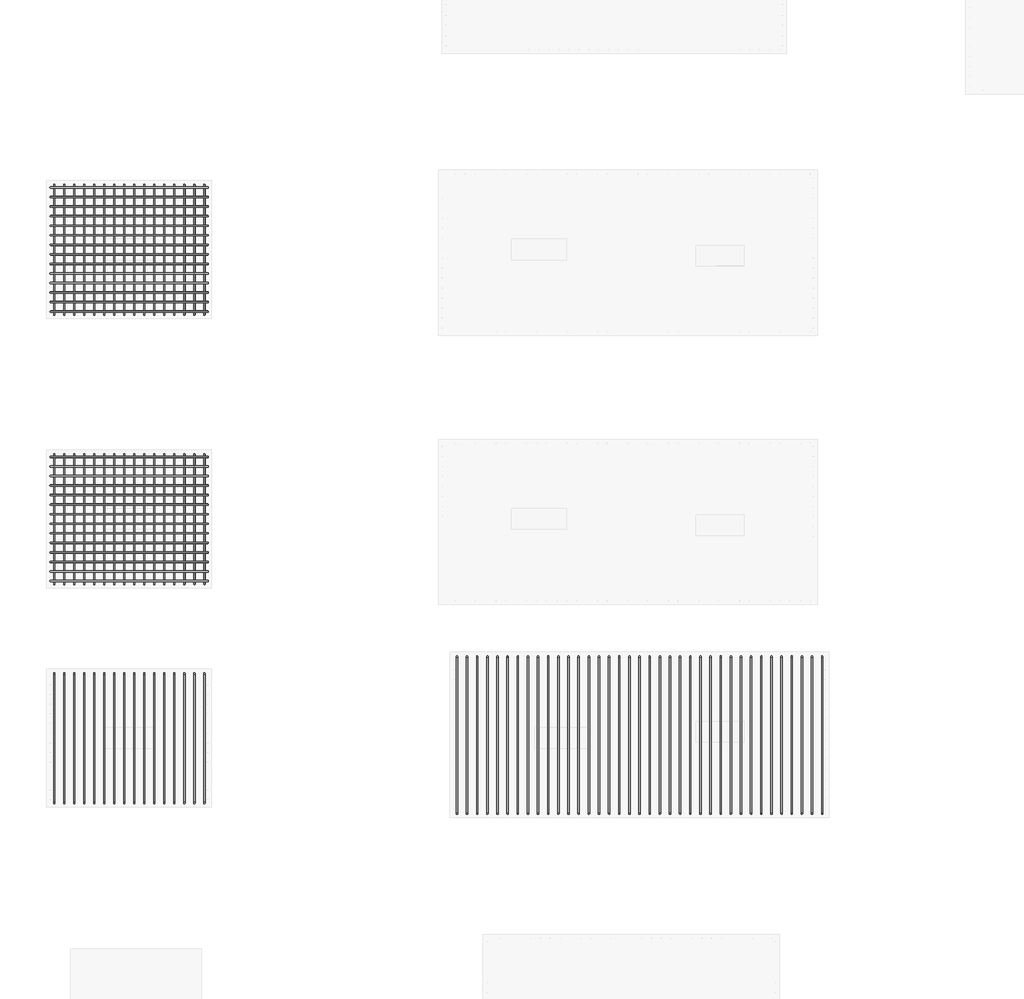
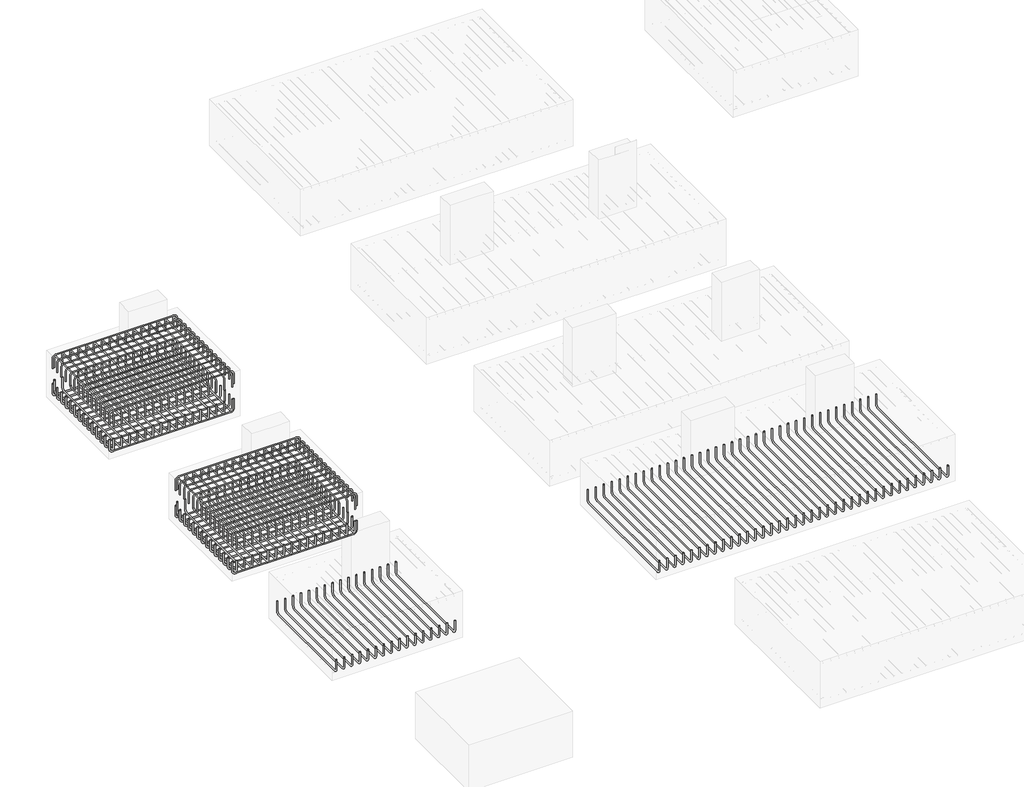
# One storey, part 4 of 21: 10 reinforcing bars.
"""IFC4 building model written with IfcOpenShell, lengths in millimetres."""

from ifc_helpers import new_model, si_unit, point, frame, origin, place, context, project, spatial, polyline, circle_curve, trimmed, segment, composite_curve, source, transform, mapped, element, save
from ifc_brep_helpers import swept_disk

model = new_model("IFC4")

# Units and contexts
model_context = context("Model", 3, world=origin())
ifc_project = project(units=[si_unit("LENGTHUNIT", "METRE", prefix="MILLI")], contexts=[model_context])

# Site, building, storey
site = spatial("IfcSite", under=ifc_project)
building = spatial("IfcBuilding", under=site)
storey = spatial("IfcBuildingStorey", under=building, Elevation=-1100.0)

# Reinforcing bars
placement = place(None, origin())
reinforcing_bar_shape = source(origin(), model_context, "Body", "SolidModel", [
    swept_disk(composite_curve([segment(polyline([(-23061.1351198, 447.9216575, -1700.0), (-23061.1351198, 447.9216575, -1882.5)]), True, "CONTINUOUS"), segment(trimmed(circle_curve(frame((-23118.6351198, 447.9216575, -1882.5), z_axis=(0.0, 1.0, 0.0), x_axis=(57.5, 0.0, 0.0)), 57.5), [point((-23061.1351198, 447.9216575, -1882.5))], [point((-23118.6351198, 447.9216575, -1940.0))], True, "CARTESIAN"), True, "CONTINUOUS"), segment(polyline([(-23118.6351198, 447.9216575, -1940.0), (-25283.6351198, 447.9216575, -1940.0)]), True, "CONTINUOUS"), segment(trimmed(circle_curve(frame((-25283.6351198, 447.9216575, -1882.5), z_axis=(0.0, 1.0, 0.0), x_axis=(0.0, 0.0, -57.5)), 57.5), [point((-25283.6351198, 447.9216575, -1940.0))], [point((-25341.1351198, 447.9216575, -1882.5))], True, "CARTESIAN"), True, "CONTINUOUS"), segment(polyline([(-25341.1351198, 447.9216575, -1882.5), (-25341.1351198, 447.9216575, -1700.0)]), True, "CONTINUOUS")], self_intersect=False), 10.0),
])
element("IfcReinforcingBar", 1, at=placement, inside=storey, context=model_context, shape_type="MappedRepresentation", body=[
    mapped(reinforcing_bar_shape, transform((0.0, 0.0, 0.0), x_axis=(1.0, 0.0, 0.0), y_axis=(0.0, 1.0, 0.0), z_axis=(0.0, 0.0, 1.0))),
    mapped(reinforcing_bar_shape, transform((0.0, -138.5928916, 0.0), x_axis=(1.0, 0.0, 0.0), y_axis=(0.0, 1.0, 0.0), z_axis=(0.0, 0.0, 1.0))),
    mapped(reinforcing_bar_shape, transform((0.0, -277.1857833, 0.0), x_axis=(1.0, 0.0, 0.0), y_axis=(0.0, 1.0, 0.0), z_axis=(0.0, 0.0, 1.0))),
    mapped(reinforcing_bar_shape, transform((0.0, -415.7786749, 0.0), x_axis=(1.0, 0.0, 0.0), y_axis=(0.0, 1.0, 0.0), z_axis=(0.0, 0.0, 1.0))),
    mapped(reinforcing_bar_shape, transform((0.0, -554.3715666, 0.0), x_axis=(1.0, 0.0, 0.0), y_axis=(0.0, 1.0, 0.0), z_axis=(0.0, 0.0, 1.0))),
    mapped(reinforcing_bar_shape, transform((0.0, -692.9644582, 0.0), x_axis=(1.0, 0.0, 0.0), y_axis=(0.0, 1.0, 0.0), z_axis=(0.0, 0.0, 1.0))),
    mapped(reinforcing_bar_shape, transform((0.0, -831.5573499, 0.0), x_axis=(1.0, 0.0, 0.0), y_axis=(0.0, 1.0, 0.0), z_axis=(0.0, 0.0, 1.0))),
    mapped(reinforcing_bar_shape, transform((0.0, -970.1502415, 0.0), x_axis=(1.0, 0.0, 0.0), y_axis=(0.0, 1.0, 0.0), z_axis=(0.0, 0.0, 1.0))),
    mapped(reinforcing_bar_shape, transform((0.0, -1108.7431331, 0.0), x_axis=(1.0, 0.0, 0.0), y_axis=(0.0, 1.0, 0.0), z_axis=(0.0, 0.0, 1.0))),
    mapped(reinforcing_bar_shape, transform((0.0, -1247.3360248, 0.0), x_axis=(1.0, 0.0, 0.0), y_axis=(0.0, 1.0, 0.0), z_axis=(0.0, 0.0, 1.0))),
    mapped(reinforcing_bar_shape, transform((0.0, -1385.9289164, 0.0), x_axis=(1.0, 0.0, 0.0), y_axis=(0.0, 1.0, 0.0), z_axis=(0.0, 0.0, 1.0))),
    mapped(reinforcing_bar_shape, transform((0.0, -1524.5218081, 0.0), x_axis=(1.0, 0.0, 0.0), y_axis=(0.0, 1.0, 0.0), z_axis=(0.0, 0.0, 1.0))),
    mapped(reinforcing_bar_shape, transform((0.0, -1663.1146997, 0.0), x_axis=(1.0, 0.0, 0.0), y_axis=(0.0, 1.0, 0.0), z_axis=(0.0, 0.0, 1.0))),
    mapped(reinforcing_bar_shape, transform((0.0, -1801.7075913, 0.0), x_axis=(1.0, 0.0, 0.0), y_axis=(0.0, 1.0, 0.0), z_axis=(0.0, 0.0, 1.0))),
])
reinforcing_bar_2_shape = source(origin(), model_context, "Body", "SolidModel", [
    swept_disk(composite_curve([segment(polyline([(-25343.1851198, 447.9216575, -1400.0), (-25343.1851198, 447.9216575, -1213.4)]), True, "CONTINUOUS"), segment(trimmed(circle_curve(frame((-25287.7351198, 447.9216575, -1213.4), z_axis=(0.0, 1.0, 0.0), x_axis=(-55.45000000000073, 0.0, 0.0)), 55.45), [point((-25343.1851198, 447.9216575, -1213.4))], [point((-25287.7351198, 447.9216575, -1157.95))], True, "CARTESIAN"), True, "CONTINUOUS"), segment(polyline([(-25287.7351198, 447.9216575, -1157.95), (-23114.5351198, 447.9216575, -1157.95)]), True, "CONTINUOUS"), segment(trimmed(circle_curve(frame((-23114.5351198, 447.9216575, -1213.4), z_axis=(0.0, 1.0, 0.0), x_axis=(0.0, 0.0, 55.450000000000045)), 55.45), [point((-23114.5351198, 447.9216575, -1157.95))], [point((-23059.0851198, 447.9216575, -1213.4))], True, "CARTESIAN"), True, "CONTINUOUS"), segment(polyline([(-23059.0851198, 447.9216575, -1213.4), (-23059.0851198, 447.9216575, -1400.0)]), True, "CONTINUOUS")], self_intersect=False), 7.95),
])
element("IfcReinforcingBar", 2, at=placement, inside=storey, context=model_context, shape_type="MappedRepresentation", body=[
    mapped(reinforcing_bar_2_shape, transform((0.0, 0.0, 0.0), x_axis=(1.0, 0.0, 0.0), y_axis=(0.0, 1.0, 0.0), z_axis=(0.0, 0.0, 1.0))),
    mapped(reinforcing_bar_2_shape, transform((0.0, -138.5928916, 0.0), x_axis=(1.0, 0.0, 0.0), y_axis=(0.0, 1.0, 0.0), z_axis=(0.0, 0.0, 1.0))),
    mapped(reinforcing_bar_2_shape, transform((0.0, -277.1857833, 0.0), x_axis=(1.0, 0.0, 0.0), y_axis=(0.0, 1.0, 0.0), z_axis=(0.0, 0.0, 1.0))),
    mapped(reinforcing_bar_2_shape, transform((0.0, -415.7786749, 0.0), x_axis=(1.0, 0.0, 0.0), y_axis=(0.0, 1.0, 0.0), z_axis=(0.0, 0.0, 1.0))),
    mapped(reinforcing_bar_2_shape, transform((0.0, -554.3715666, 0.0), x_axis=(1.0, 0.0, 0.0), y_axis=(0.0, 1.0, 0.0), z_axis=(0.0, 0.0, 1.0))),
    mapped(reinforcing_bar_2_shape, transform((0.0, -692.9644582, 0.0), x_axis=(1.0, 0.0, 0.0), y_axis=(0.0, 1.0, 0.0), z_axis=(0.0, 0.0, 1.0))),
    mapped(reinforcing_bar_2_shape, transform((0.0, -831.5573499, 0.0), x_axis=(1.0, 0.0, 0.0), y_axis=(0.0, 1.0, 0.0), z_axis=(0.0, 0.0, 1.0))),
    mapped(reinforcing_bar_2_shape, transform((0.0, -970.1502415, 0.0), x_axis=(1.0, 0.0, 0.0), y_axis=(0.0, 1.0, 0.0), z_axis=(0.0, 0.0, 1.0))),
    mapped(reinforcing_bar_2_shape, transform((0.0, -1108.7431331, 0.0), x_axis=(1.0, 0.0, 0.0), y_axis=(0.0, 1.0, 0.0), z_axis=(0.0, 0.0, 1.0))),
    mapped(reinforcing_bar_2_shape, transform((0.0, -1247.3360248, 0.0), x_axis=(1.0, 0.0, 0.0), y_axis=(0.0, 1.0, 0.0), z_axis=(0.0, 0.0, 1.0))),
    mapped(reinforcing_bar_2_shape, transform((0.0, -1385.9289164, 0.0), x_axis=(1.0, 0.0, 0.0), y_axis=(0.0, 1.0, 0.0), z_axis=(0.0, 0.0, 1.0))),
    mapped(reinforcing_bar_2_shape, transform((0.0, -1524.5218081, 0.0), x_axis=(1.0, 0.0, 0.0), y_axis=(0.0, 1.0, 0.0), z_axis=(0.0, 0.0, 1.0))),
    mapped(reinforcing_bar_2_shape, transform((0.0, -1663.1146997, 0.0), x_axis=(1.0, 0.0, 0.0), y_axis=(0.0, 1.0, 0.0), z_axis=(0.0, 0.0, 1.0))),
    mapped(reinforcing_bar_2_shape, transform((0.0, -1801.7075913, 0.0), x_axis=(1.0, 0.0, 0.0), y_axis=(0.0, 1.0, 0.0), z_axis=(0.0, 0.0, 1.0))),
])
reinforcing_bar_3_shape = source(origin(), model_context, "Body", "SolidModel", [
    swept_disk(composite_curve([segment(polyline([(-23110.9192838, 486.2204288, -1428.1111113), (-23110.9192838, 486.2204288, -1241.5111113)]), True, "CONTINUOUS"), segment(trimmed(circle_curve(frame((-23110.9192838, 430.7704288, -1241.5111113), z_axis=(1.0, 0.0, 0.0), x_axis=(0.0, 55.44999999999999, 0.0)), 55.45), [point((-23110.9192838, 486.2204288, -1241.5111113))], [point((-23110.9192838, 430.7704288, -1186.0611113))], True, "CARTESIAN"), True, "CONTINUOUS"), segment(polyline([(-23110.9192838, 430.7704288, -1186.0611113), (-23110.9192838, -1342.4295712, -1186.0611113)]), True, "CONTINUOUS"), segment(trimmed(circle_curve(frame((-23110.9192838, -1342.4295712, -1241.5111113), z_axis=(1.0, 0.0, 0.0), x_axis=(0.0, 0.0, 55.450000000000045)), 55.45), [point((-23110.9192838, -1342.4295712, -1186.0611113))], [point((-23110.9192838, -1397.8795712, -1241.5111113))], True, "CARTESIAN"), True, "CONTINUOUS"), segment(polyline([(-23110.9192838, -1397.8795712, -1241.5111113), (-23110.9192838, -1397.8795712, -1428.1111113)]), True, "CONTINUOUS")], self_intersect=False), 7.95),
])
element("IfcReinforcingBar", 3, at=placement, inside=storey, context=model_context, shape_type="MappedRepresentation", body=[
    mapped(reinforcing_bar_3_shape, transform((0.0, 0.0, 0.0), x_axis=(1.0, 0.0, 0.0), y_axis=(0.0, 1.0, 0.0), z_axis=(0.0, 0.0, 1.0))),
    mapped(reinforcing_bar_3_shape, transform((-145.2528929, 0.0, 0.0), x_axis=(1.0, 0.0, 0.0), y_axis=(0.0, 1.0, 0.0), z_axis=(0.0, 0.0, 1.0))),
    mapped(reinforcing_bar_3_shape, transform((-290.5057858, 0.0, 0.0), x_axis=(1.0, 0.0, 0.0), y_axis=(0.0, 1.0, 0.0), z_axis=(0.0, 0.0, 1.0))),
    mapped(reinforcing_bar_3_shape, transform((-435.7586787, 0.0, 0.0), x_axis=(1.0, 0.0, 0.0), y_axis=(0.0, 1.0, 0.0), z_axis=(0.0, 0.0, 1.0))),
    mapped(reinforcing_bar_3_shape, transform((-581.0115716, 0.0, 0.0), x_axis=(1.0, 0.0, 0.0), y_axis=(0.0, 1.0, 0.0), z_axis=(0.0, 0.0, 1.0))),
    mapped(reinforcing_bar_3_shape, transform((-726.2644645, 0.0, 0.0), x_axis=(1.0, 0.0, 0.0), y_axis=(0.0, 1.0, 0.0), z_axis=(0.0, 0.0, 1.0))),
    mapped(reinforcing_bar_3_shape, transform((-871.5173574, 0.0, 0.0), x_axis=(1.0, 0.0, 0.0), y_axis=(0.0, 1.0, 0.0), z_axis=(0.0, 0.0, 1.0))),
    mapped(reinforcing_bar_3_shape, transform((-1016.7702503, 0.0, 0.0), x_axis=(1.0, 0.0, 0.0), y_axis=(0.0, 1.0, 0.0), z_axis=(0.0, 0.0, 1.0))),
    mapped(reinforcing_bar_3_shape, transform((-1162.0231432, 0.0, 0.0), x_axis=(1.0, 0.0, 0.0), y_axis=(0.0, 1.0, 0.0), z_axis=(0.0, 0.0, 1.0))),
    mapped(reinforcing_bar_3_shape, transform((-1307.276036, 0.0, 0.0), x_axis=(1.0, 0.0, 0.0), y_axis=(0.0, 1.0, 0.0), z_axis=(0.0, 0.0, 1.0))),
    mapped(reinforcing_bar_3_shape, transform((-1452.5289289, 0.0, 0.0), x_axis=(1.0, 0.0, 0.0), y_axis=(0.0, 1.0, 0.0), z_axis=(0.0, 0.0, 1.0))),
    mapped(reinforcing_bar_3_shape, transform((-1597.7818218, 0.0, 0.0), x_axis=(1.0, 0.0, 0.0), y_axis=(0.0, 1.0, 0.0), z_axis=(0.0, 0.0, 1.0))),
    mapped(reinforcing_bar_3_shape, transform((-1743.0347147, 0.0, 0.0), x_axis=(1.0, 0.0, 0.0), y_axis=(0.0, 1.0, 0.0), z_axis=(0.0, 0.0, 1.0))),
    mapped(reinforcing_bar_3_shape, transform((-1888.2876076, 0.0, 0.0), x_axis=(1.0, 0.0, 0.0), y_axis=(0.0, 1.0, 0.0), z_axis=(0.0, 0.0, 1.0))),
    mapped(reinforcing_bar_3_shape, transform((-2033.5405005, 0.0, 0.0), x_axis=(1.0, 0.0, 0.0), y_axis=(0.0, 1.0, 0.0), z_axis=(0.0, 0.0, 1.0))),
    mapped(reinforcing_bar_3_shape, transform((-2178.7933934, 0.0, 0.0), x_axis=(1.0, 0.0, 0.0), y_axis=(0.0, 1.0, 0.0), z_axis=(0.0, 0.0, 1.0))),
])
reinforcing_bar_4_shape = source(origin(), model_context, "Body", "SolidModel", [
    swept_disk(composite_curve([segment(polyline([(-25289.7126773, 484.1704288, -1669.8442859), (-25289.7126773, 484.1704288, -1852.3442859)]), True, "CONTINUOUS"), segment(trimmed(circle_curve(frame((-25289.7126773, 426.6704288, -1852.3442859), z_axis=(-1.0, 0.0, 0.0), x_axis=(0.0, 57.5, 0.0)), 57.5), [point((-25289.7126773, 484.1704288, -1852.3442859))], [point((-25289.7126773, 426.6704288, -1909.8442859))], True, "CARTESIAN"), True, "CONTINUOUS"), segment(polyline([(-25289.7126773, 426.6704288, -1909.8442859), (-25289.7126773, -1338.3295712, -1909.8442859)]), True, "CONTINUOUS"), segment(trimmed(circle_curve(frame((-25289.7126773, -1338.3295712, -1852.3442859), z_axis=(-1.0, 0.0, 0.0), x_axis=(0.0, 0.0, -57.5)), 57.5), [point((-25289.7126773, -1338.3295712, -1909.8442859))], [point((-25289.7126773, -1395.8295712, -1852.3442859))], True, "CARTESIAN"), True, "CONTINUOUS"), segment(polyline([(-25289.7126773, -1395.8295712, -1852.3442859), (-25289.7126773, -1395.8295712, -1669.8442859)]), True, "CONTINUOUS")], self_intersect=False), 10.0),
])
element("IfcReinforcingBar", 4, at=placement, inside=storey, context=model_context, shape_type="MappedRepresentation", body=[
    mapped(reinforcing_bar_4_shape, transform((0.0, 0.0, 0.0), x_axis=(1.0, 0.0, 0.0), y_axis=(0.0, 1.0, 0.0), z_axis=(0.0, 0.0, 1.0))),
    mapped(reinforcing_bar_4_shape, transform((145.2528929, 0.0, 0.0), x_axis=(1.0, 0.0, 0.0), y_axis=(0.0, 1.0, 0.0), z_axis=(0.0, 0.0, 1.0))),
    mapped(reinforcing_bar_4_shape, transform((290.5057858, 0.0, 0.0), x_axis=(1.0, 0.0, 0.0), y_axis=(0.0, 1.0, 0.0), z_axis=(0.0, 0.0, 1.0))),
    mapped(reinforcing_bar_4_shape, transform((435.7586787, 0.0, 0.0), x_axis=(1.0, 0.0, 0.0), y_axis=(0.0, 1.0, 0.0), z_axis=(0.0, 0.0, 1.0))),
    mapped(reinforcing_bar_4_shape, transform((581.0115716, 0.0, 0.0), x_axis=(1.0, 0.0, 0.0), y_axis=(0.0, 1.0, 0.0), z_axis=(0.0, 0.0, 1.0))),
    mapped(reinforcing_bar_4_shape, transform((726.2644645, 0.0, 0.0), x_axis=(1.0, 0.0, 0.0), y_axis=(0.0, 1.0, 0.0), z_axis=(0.0, 0.0, 1.0))),
    mapped(reinforcing_bar_4_shape, transform((871.5173574, 0.0, 0.0), x_axis=(1.0, 0.0, 0.0), y_axis=(0.0, 1.0, 0.0), z_axis=(0.0, 0.0, 1.0))),
    mapped(reinforcing_bar_4_shape, transform((1016.7702503, 0.0, 0.0), x_axis=(1.0, 0.0, 0.0), y_axis=(0.0, 1.0, 0.0), z_axis=(0.0, 0.0, 1.0))),
    mapped(reinforcing_bar_4_shape, transform((1162.0231432, 0.0, 0.0), x_axis=(1.0, 0.0, 0.0), y_axis=(0.0, 1.0, 0.0), z_axis=(0.0, 0.0, 1.0))),
    mapped(reinforcing_bar_4_shape, transform((1307.276036, 0.0, 0.0), x_axis=(1.0, 0.0, 0.0), y_axis=(0.0, 1.0, 0.0), z_axis=(0.0, 0.0, 1.0))),
    mapped(reinforcing_bar_4_shape, transform((1452.5289289, 0.0, 0.0), x_axis=(1.0, 0.0, 0.0), y_axis=(0.0, 1.0, 0.0), z_axis=(0.0, 0.0, 1.0))),
    mapped(reinforcing_bar_4_shape, transform((1597.7818218, 0.0, 0.0), x_axis=(1.0, 0.0, 0.0), y_axis=(0.0, 1.0, 0.0), z_axis=(0.0, 0.0, 1.0))),
    mapped(reinforcing_bar_4_shape, transform((1743.0347147, 0.0, 0.0), x_axis=(1.0, 0.0, 0.0), y_axis=(0.0, 1.0, 0.0), z_axis=(0.0, 0.0, 1.0))),
    mapped(reinforcing_bar_4_shape, transform((1888.2876076, 0.0, 0.0), x_axis=(1.0, 0.0, 0.0), y_axis=(0.0, 1.0, 0.0), z_axis=(0.0, 0.0, 1.0))),
    mapped(reinforcing_bar_4_shape, transform((2033.5405005, 0.0, 0.0), x_axis=(1.0, 0.0, 0.0), y_axis=(0.0, 1.0, 0.0), z_axis=(0.0, 0.0, 1.0))),
    mapped(reinforcing_bar_4_shape, transform((2178.7933934, 0.0, 0.0), x_axis=(1.0, 0.0, 0.0), y_axis=(0.0, 1.0, 0.0), z_axis=(0.0, 0.0, 1.0))),
])
reinforcing_bar_5_shape = source(origin(), model_context, "Body", "SolidModel", [
    swept_disk(composite_curve([segment(polyline([(-23061.1351198, -3462.0783425, -1700.0), (-23061.1351198, -3462.0783425, -1882.5)]), True, "CONTINUOUS"), segment(trimmed(circle_curve(frame((-23118.6351198, -3462.0783425, -1882.5), z_axis=(0.0, 1.0, 0.0), x_axis=(57.5, 0.0, 0.0)), 57.5), [point((-23061.1351198, -3462.0783425, -1882.5))], [point((-23118.6351198, -3462.0783425, -1940.0))], True, "CARTESIAN"), True, "CONTINUOUS"), segment(polyline([(-23118.6351198, -3462.0783425, -1940.0), (-25283.6351198, -3462.0783425, -1940.0)]), True, "CONTINUOUS"), segment(trimmed(circle_curve(frame((-25283.6351198, -3462.0783425, -1882.5), z_axis=(0.0, 1.0, 0.0), x_axis=(0.0, 0.0, -57.5)), 57.5), [point((-25283.6351198, -3462.0783425, -1940.0))], [point((-25341.1351198, -3462.0783425, -1882.5))], True, "CARTESIAN"), True, "CONTINUOUS"), segment(polyline([(-25341.1351198, -3462.0783425, -1882.5), (-25341.1351198, -3462.0783425, -1700.0)]), True, "CONTINUOUS")], self_intersect=False), 10.0),
])
element("IfcReinforcingBar", 5, at=placement, inside=storey, context=model_context, shape_type="MappedRepresentation", body=[
    mapped(reinforcing_bar_5_shape, transform((0.0, 0.0, 0.0), x_axis=(1.0, 0.0, 0.0), y_axis=(0.0, 1.0, 0.0), z_axis=(0.0, 0.0, 1.0))),
    mapped(reinforcing_bar_5_shape, transform((0.0, -138.5928916, 0.0), x_axis=(1.0, 0.0, 0.0), y_axis=(0.0, 1.0, 0.0), z_axis=(0.0, 0.0, 1.0))),
    mapped(reinforcing_bar_5_shape, transform((0.0, -277.1857833, 0.0), x_axis=(1.0, 0.0, 0.0), y_axis=(0.0, 1.0, 0.0), z_axis=(0.0, 0.0, 1.0))),
    mapped(reinforcing_bar_5_shape, transform((0.0, -415.7786749, 0.0), x_axis=(1.0, 0.0, 0.0), y_axis=(0.0, 1.0, 0.0), z_axis=(0.0, 0.0, 1.0))),
    mapped(reinforcing_bar_5_shape, transform((0.0, -554.3715666, 0.0), x_axis=(1.0, 0.0, 0.0), y_axis=(0.0, 1.0, 0.0), z_axis=(0.0, 0.0, 1.0))),
    mapped(reinforcing_bar_5_shape, transform((0.0, -692.9644582, 0.0), x_axis=(1.0, 0.0, 0.0), y_axis=(0.0, 1.0, 0.0), z_axis=(0.0, 0.0, 1.0))),
    mapped(reinforcing_bar_5_shape, transform((0.0, -831.5573499, 0.0), x_axis=(1.0, 0.0, 0.0), y_axis=(0.0, 1.0, 0.0), z_axis=(0.0, 0.0, 1.0))),
    mapped(reinforcing_bar_5_shape, transform((0.0, -970.1502415, 0.0), x_axis=(1.0, 0.0, 0.0), y_axis=(0.0, 1.0, 0.0), z_axis=(0.0, 0.0, 1.0))),
    mapped(reinforcing_bar_5_shape, transform((0.0, -1108.7431331, 0.0), x_axis=(1.0, 0.0, 0.0), y_axis=(0.0, 1.0, 0.0), z_axis=(0.0, 0.0, 1.0))),
    mapped(reinforcing_bar_5_shape, transform((0.0, -1247.3360248, 0.0), x_axis=(1.0, 0.0, 0.0), y_axis=(0.0, 1.0, 0.0), z_axis=(0.0, 0.0, 1.0))),
    mapped(reinforcing_bar_5_shape, transform((0.0, -1385.9289164, 0.0), x_axis=(1.0, 0.0, 0.0), y_axis=(0.0, 1.0, 0.0), z_axis=(0.0, 0.0, 1.0))),
    mapped(reinforcing_bar_5_shape, transform((0.0, -1524.5218081, 0.0), x_axis=(1.0, 0.0, 0.0), y_axis=(0.0, 1.0, 0.0), z_axis=(0.0, 0.0, 1.0))),
    mapped(reinforcing_bar_5_shape, transform((0.0, -1663.1146997, 0.0), x_axis=(1.0, 0.0, 0.0), y_axis=(0.0, 1.0, 0.0), z_axis=(0.0, 0.0, 1.0))),
    mapped(reinforcing_bar_5_shape, transform((0.0, -1801.7075913, 0.0), x_axis=(1.0, 0.0, 0.0), y_axis=(0.0, 1.0, 0.0), z_axis=(0.0, 0.0, 1.0))),
])
reinforcing_bar_6_shape = source(origin(), model_context, "Body", "SolidModel", [
    swept_disk(composite_curve([segment(polyline([(-25343.1851198, -3462.0783425, -1400.0), (-25343.1851198, -3462.0783425, -1213.4)]), True, "CONTINUOUS"), segment(trimmed(circle_curve(frame((-25287.7351198, -3462.0783425, -1213.4), z_axis=(0.0, 1.0, 0.0), x_axis=(-55.45000000000073, 0.0, 0.0)), 55.45), [point((-25343.1851198, -3462.0783425, -1213.4))], [point((-25287.7351198, -3462.0783425, -1157.95))], True, "CARTESIAN"), True, "CONTINUOUS"), segment(polyline([(-25287.7351198, -3462.0783425, -1157.95), (-23114.5351198, -3462.0783425, -1157.95)]), True, "CONTINUOUS"), segment(trimmed(circle_curve(frame((-23114.5351198, -3462.0783425, -1213.4), z_axis=(0.0, 1.0, 0.0), x_axis=(0.0, 0.0, 55.450000000000045)), 55.45), [point((-23114.5351198, -3462.0783425, -1157.95))], [point((-23059.0851198, -3462.0783425, -1213.4))], True, "CARTESIAN"), True, "CONTINUOUS"), segment(polyline([(-23059.0851198, -3462.0783425, -1213.4), (-23059.0851198, -3462.0783425, -1400.0)]), True, "CONTINUOUS")], self_intersect=False), 7.95),
])
element("IfcReinforcingBar", 6, at=placement, inside=storey, context=model_context, shape_type="MappedRepresentation", body=[
    mapped(reinforcing_bar_6_shape, transform((0.0, 0.0, 0.0), x_axis=(1.0, 0.0, 0.0), y_axis=(0.0, 1.0, 0.0), z_axis=(0.0, 0.0, 1.0))),
    mapped(reinforcing_bar_6_shape, transform((0.0, -138.5928916, 0.0), x_axis=(1.0, 0.0, 0.0), y_axis=(0.0, 1.0, 0.0), z_axis=(0.0, 0.0, 1.0))),
    mapped(reinforcing_bar_6_shape, transform((0.0, -277.1857833, 0.0), x_axis=(1.0, 0.0, 0.0), y_axis=(0.0, 1.0, 0.0), z_axis=(0.0, 0.0, 1.0))),
    mapped(reinforcing_bar_6_shape, transform((0.0, -415.7786749, 0.0), x_axis=(1.0, 0.0, 0.0), y_axis=(0.0, 1.0, 0.0), z_axis=(0.0, 0.0, 1.0))),
    mapped(reinforcing_bar_6_shape, transform((0.0, -554.3715666, 0.0), x_axis=(1.0, 0.0, 0.0), y_axis=(0.0, 1.0, 0.0), z_axis=(0.0, 0.0, 1.0))),
    mapped(reinforcing_bar_6_shape, transform((0.0, -692.9644582, 0.0), x_axis=(1.0, 0.0, 0.0), y_axis=(0.0, 1.0, 0.0), z_axis=(0.0, 0.0, 1.0))),
    mapped(reinforcing_bar_6_shape, transform((0.0, -831.5573499, 0.0), x_axis=(1.0, 0.0, 0.0), y_axis=(0.0, 1.0, 0.0), z_axis=(0.0, 0.0, 1.0))),
    mapped(reinforcing_bar_6_shape, transform((0.0, -970.1502415, 0.0), x_axis=(1.0, 0.0, 0.0), y_axis=(0.0, 1.0, 0.0), z_axis=(0.0, 0.0, 1.0))),
    mapped(reinforcing_bar_6_shape, transform((0.0, -1108.7431331, 0.0), x_axis=(1.0, 0.0, 0.0), y_axis=(0.0, 1.0, 0.0), z_axis=(0.0, 0.0, 1.0))),
    mapped(reinforcing_bar_6_shape, transform((0.0, -1247.3360248, 0.0), x_axis=(1.0, 0.0, 0.0), y_axis=(0.0, 1.0, 0.0), z_axis=(0.0, 0.0, 1.0))),
    mapped(reinforcing_bar_6_shape, transform((0.0, -1385.9289164, 0.0), x_axis=(1.0, 0.0, 0.0), y_axis=(0.0, 1.0, 0.0), z_axis=(0.0, 0.0, 1.0))),
    mapped(reinforcing_bar_6_shape, transform((0.0, -1524.5218081, 0.0), x_axis=(1.0, 0.0, 0.0), y_axis=(0.0, 1.0, 0.0), z_axis=(0.0, 0.0, 1.0))),
    mapped(reinforcing_bar_6_shape, transform((0.0, -1663.1146997, 0.0), x_axis=(1.0, 0.0, 0.0), y_axis=(0.0, 1.0, 0.0), z_axis=(0.0, 0.0, 1.0))),
    mapped(reinforcing_bar_6_shape, transform((0.0, -1801.7075913, 0.0), x_axis=(1.0, 0.0, 0.0), y_axis=(0.0, 1.0, 0.0), z_axis=(0.0, 0.0, 1.0))),
])
reinforcing_bar_7_shape = source(origin(), model_context, "Body", "SolidModel", [
    swept_disk(composite_curve([segment(polyline([(-23110.9192838, -3423.7795712, -1428.1111113), (-23110.9192838, -3423.7795712, -1241.5111113)]), True, "CONTINUOUS"), segment(trimmed(circle_curve(frame((-23110.9192838, -3479.2295712, -1241.5111113), z_axis=(1.0, 0.0, 0.0), x_axis=(0.0, 55.44999999999982, 0.0)), 55.45), [point((-23110.9192838, -3423.7795712, -1241.5111113))], [point((-23110.9192838, -3479.2295712, -1186.0611113))], True, "CARTESIAN"), True, "CONTINUOUS"), segment(polyline([(-23110.9192838, -3479.2295712, -1186.0611113), (-23110.9192838, -5252.4295712, -1186.0611113)]), True, "CONTINUOUS"), segment(trimmed(circle_curve(frame((-23110.9192838, -5252.4295712, -1241.5111113), z_axis=(1.0, 0.0, 0.0), x_axis=(0.0, 0.0, 55.450000000000045)), 55.45), [point((-23110.9192838, -5252.4295712, -1186.0611113))], [point((-23110.9192838, -5307.8795712, -1241.5111113))], True, "CARTESIAN"), True, "CONTINUOUS"), segment(polyline([(-23110.9192838, -5307.8795712, -1241.5111113), (-23110.9192838, -5307.8795712, -1428.1111113)]), True, "CONTINUOUS")], self_intersect=False), 7.95),
])
element("IfcReinforcingBar", 7, at=placement, inside=storey, context=model_context, shape_type="MappedRepresentation", body=[
    mapped(reinforcing_bar_7_shape, transform((0.0, 0.0, 0.0), x_axis=(1.0, 0.0, 0.0), y_axis=(0.0, 1.0, 0.0), z_axis=(0.0, 0.0, 1.0))),
    mapped(reinforcing_bar_7_shape, transform((-145.2528929, 0.0, 0.0), x_axis=(1.0, 0.0, 0.0), y_axis=(0.0, 1.0, 0.0), z_axis=(0.0, 0.0, 1.0))),
    mapped(reinforcing_bar_7_shape, transform((-290.5057858, 0.0, 0.0), x_axis=(1.0, 0.0, 0.0), y_axis=(0.0, 1.0, 0.0), z_axis=(0.0, 0.0, 1.0))),
    mapped(reinforcing_bar_7_shape, transform((-435.7586787, 0.0, 0.0), x_axis=(1.0, 0.0, 0.0), y_axis=(0.0, 1.0, 0.0), z_axis=(0.0, 0.0, 1.0))),
    mapped(reinforcing_bar_7_shape, transform((-581.0115716, 0.0, 0.0), x_axis=(1.0, 0.0, 0.0), y_axis=(0.0, 1.0, 0.0), z_axis=(0.0, 0.0, 1.0))),
    mapped(reinforcing_bar_7_shape, transform((-726.2644645, 0.0, 0.0), x_axis=(1.0, 0.0, 0.0), y_axis=(0.0, 1.0, 0.0), z_axis=(0.0, 0.0, 1.0))),
    mapped(reinforcing_bar_7_shape, transform((-871.5173574, 0.0, 0.0), x_axis=(1.0, 0.0, 0.0), y_axis=(0.0, 1.0, 0.0), z_axis=(0.0, 0.0, 1.0))),
    mapped(reinforcing_bar_7_shape, transform((-1016.7702503, 0.0, 0.0), x_axis=(1.0, 0.0, 0.0), y_axis=(0.0, 1.0, 0.0), z_axis=(0.0, 0.0, 1.0))),
    mapped(reinforcing_bar_7_shape, transform((-1162.0231432, 0.0, 0.0), x_axis=(1.0, 0.0, 0.0), y_axis=(0.0, 1.0, 0.0), z_axis=(0.0, 0.0, 1.0))),
    mapped(reinforcing_bar_7_shape, transform((-1307.276036, 0.0, 0.0), x_axis=(1.0, 0.0, 0.0), y_axis=(0.0, 1.0, 0.0), z_axis=(0.0, 0.0, 1.0))),
    mapped(reinforcing_bar_7_shape, transform((-1452.5289289, 0.0, 0.0), x_axis=(1.0, 0.0, 0.0), y_axis=(0.0, 1.0, 0.0), z_axis=(0.0, 0.0, 1.0))),
    mapped(reinforcing_bar_7_shape, transform((-1597.7818218, 0.0, 0.0), x_axis=(1.0, 0.0, 0.0), y_axis=(0.0, 1.0, 0.0), z_axis=(0.0, 0.0, 1.0))),
    mapped(reinforcing_bar_7_shape, transform((-1743.0347147, 0.0, 0.0), x_axis=(1.0, 0.0, 0.0), y_axis=(0.0, 1.0, 0.0), z_axis=(0.0, 0.0, 1.0))),
    mapped(reinforcing_bar_7_shape, transform((-1888.2876076, 0.0, 0.0), x_axis=(1.0, 0.0, 0.0), y_axis=(0.0, 1.0, 0.0), z_axis=(0.0, 0.0, 1.0))),
    mapped(reinforcing_bar_7_shape, transform((-2033.5405005, 0.0, 0.0), x_axis=(1.0, 0.0, 0.0), y_axis=(0.0, 1.0, 0.0), z_axis=(0.0, 0.0, 1.0))),
    mapped(reinforcing_bar_7_shape, transform((-2178.7933934, 0.0, 0.0), x_axis=(1.0, 0.0, 0.0), y_axis=(0.0, 1.0, 0.0), z_axis=(0.0, 0.0, 1.0))),
])
reinforcing_bar_8_shape = source(origin(), model_context, "Body", "SolidModel", [
    swept_disk(composite_curve([segment(polyline([(-25289.7126773, -3425.8295712, -1669.8442859), (-25289.7126773, -3425.8295712, -1852.3442859)]), True, "CONTINUOUS"), segment(trimmed(circle_curve(frame((-25289.7126773, -3483.3295712, -1852.3442859), z_axis=(-1.0, 0.0, 0.0), x_axis=(0.0, 57.5, 0.0)), 57.5), [point((-25289.7126773, -3425.8295712, -1852.3442859))], [point((-25289.7126773, -3483.3295712, -1909.8442859))], True, "CARTESIAN"), True, "CONTINUOUS"), segment(polyline([(-25289.7126773, -3483.3295712, -1909.8442859), (-25289.7126773, -5248.3295712, -1909.8442859)]), True, "CONTINUOUS"), segment(trimmed(circle_curve(frame((-25289.7126773, -5248.3295712, -1852.3442859), z_axis=(-1.0, 0.0, 0.0), x_axis=(0.0, 0.0, -57.5)), 57.5), [point((-25289.7126773, -5248.3295712, -1909.8442859))], [point((-25289.7126773, -5305.8295712, -1852.3442859))], True, "CARTESIAN"), True, "CONTINUOUS"), segment(polyline([(-25289.7126773, -5305.8295712, -1852.3442859), (-25289.7126773, -5305.8295712, -1669.8442859)]), True, "CONTINUOUS")], self_intersect=False), 10.0),
])
element("IfcReinforcingBar", 8, at=placement, inside=storey, context=model_context, shape_type="MappedRepresentation", body=[
    mapped(reinforcing_bar_8_shape, transform((0.0, 0.0, 0.0), x_axis=(1.0, 0.0, 0.0), y_axis=(0.0, 1.0, 0.0), z_axis=(0.0, 0.0, 1.0))),
    mapped(reinforcing_bar_8_shape, transform((145.2528929, 0.0, 0.0), x_axis=(1.0, 0.0, 0.0), y_axis=(0.0, 1.0, 0.0), z_axis=(0.0, 0.0, 1.0))),
    mapped(reinforcing_bar_8_shape, transform((290.5057858, 0.0, 0.0), x_axis=(1.0, 0.0, 0.0), y_axis=(0.0, 1.0, 0.0), z_axis=(0.0, 0.0, 1.0))),
    mapped(reinforcing_bar_8_shape, transform((435.7586787, 0.0, 0.0), x_axis=(1.0, 0.0, 0.0), y_axis=(0.0, 1.0, 0.0), z_axis=(0.0, 0.0, 1.0))),
    mapped(reinforcing_bar_8_shape, transform((581.0115716, 0.0, 0.0), x_axis=(1.0, 0.0, 0.0), y_axis=(0.0, 1.0, 0.0), z_axis=(0.0, 0.0, 1.0))),
    mapped(reinforcing_bar_8_shape, transform((726.2644645, 0.0, 0.0), x_axis=(1.0, 0.0, 0.0), y_axis=(0.0, 1.0, 0.0), z_axis=(0.0, 0.0, 1.0))),
    mapped(reinforcing_bar_8_shape, transform((871.5173574, 0.0, 0.0), x_axis=(1.0, 0.0, 0.0), y_axis=(0.0, 1.0, 0.0), z_axis=(0.0, 0.0, 1.0))),
    mapped(reinforcing_bar_8_shape, transform((1016.7702503, 0.0, 0.0), x_axis=(1.0, 0.0, 0.0), y_axis=(0.0, 1.0, 0.0), z_axis=(0.0, 0.0, 1.0))),
    mapped(reinforcing_bar_8_shape, transform((1162.0231432, 0.0, 0.0), x_axis=(1.0, 0.0, 0.0), y_axis=(0.0, 1.0, 0.0), z_axis=(0.0, 0.0, 1.0))),
    mapped(reinforcing_bar_8_shape, transform((1307.276036, 0.0, 0.0), x_axis=(1.0, 0.0, 0.0), y_axis=(0.0, 1.0, 0.0), z_axis=(0.0, 0.0, 1.0))),
    mapped(reinforcing_bar_8_shape, transform((1452.5289289, 0.0, 0.0), x_axis=(1.0, 0.0, 0.0), y_axis=(0.0, 1.0, 0.0), z_axis=(0.0, 0.0, 1.0))),
    mapped(reinforcing_bar_8_shape, transform((1597.7818218, 0.0, 0.0), x_axis=(1.0, 0.0, 0.0), y_axis=(0.0, 1.0, 0.0), z_axis=(0.0, 0.0, 1.0))),
    mapped(reinforcing_bar_8_shape, transform((1743.0347147, 0.0, 0.0), x_axis=(1.0, 0.0, 0.0), y_axis=(0.0, 1.0, 0.0), z_axis=(0.0, 0.0, 1.0))),
    mapped(reinforcing_bar_8_shape, transform((1888.2876076, 0.0, 0.0), x_axis=(1.0, 0.0, 0.0), y_axis=(0.0, 1.0, 0.0), z_axis=(0.0, 0.0, 1.0))),
    mapped(reinforcing_bar_8_shape, transform((2033.5405005, 0.0, 0.0), x_axis=(1.0, 0.0, 0.0), y_axis=(0.0, 1.0, 0.0), z_axis=(0.0, 0.0, 1.0))),
    mapped(reinforcing_bar_8_shape, transform((2178.7933934, 0.0, 0.0), x_axis=(1.0, 0.0, 0.0), y_axis=(0.0, 1.0, 0.0), z_axis=(0.0, 0.0, 1.0))),
])
reinforcing_bar_9_shape = source(origin(), model_context, "Body", "SolidModel", [
    swept_disk(composite_curve([segment(polyline([(-25289.7126773, -6605.8295712, -1669.8442859), (-25289.7126773, -6605.8295712, -1852.3442859)]), True, "CONTINUOUS"), segment(trimmed(circle_curve(frame((-25289.7126773, -6663.3295712, -1852.3442859), z_axis=(-1.0, 0.0, 0.0), x_axis=(0.0, 57.5, 0.0)), 57.5), [point((-25289.7126773, -6605.8295712, -1852.3442859))], [point((-25289.7126773, -6663.3295712, -1909.8442859))], True, "CARTESIAN"), True, "CONTINUOUS"), segment(polyline([(-25289.7126773, -6663.3295712, -1909.8442859), (-25289.7126773, -8428.3295712, -1909.8442859)]), True, "CONTINUOUS"), segment(trimmed(circle_curve(frame((-25289.7126773, -8428.3295712, -1852.3442859), z_axis=(-1.0, 0.0, 0.0), x_axis=(0.0, 0.0, -57.5)), 57.5), [point((-25289.7126773, -8428.3295712, -1909.8442859))], [point((-25289.7126773, -8485.8295712, -1852.3442859))], True, "CARTESIAN"), True, "CONTINUOUS"), segment(polyline([(-25289.7126773, -8485.8295712, -1852.3442859), (-25289.7126773, -8485.8295712, -1669.8442859)]), True, "CONTINUOUS")], self_intersect=False), 10.0),
])
element("IfcReinforcingBar", 9, at=placement, inside=storey, context=model_context, shape_type="MappedRepresentation", body=[
    mapped(reinforcing_bar_9_shape, transform((0.0, 0.0, 0.0), x_axis=(1.0, 0.0, 0.0), y_axis=(0.0, 1.0, 0.0), z_axis=(0.0, 0.0, 1.0))),
    mapped(reinforcing_bar_9_shape, transform((145.2528929, 0.0, 0.0), x_axis=(1.0, 0.0, 0.0), y_axis=(0.0, 1.0, 0.0), z_axis=(0.0, 0.0, 1.0))),
    mapped(reinforcing_bar_9_shape, transform((290.5057858, 0.0, 0.0), x_axis=(1.0, 0.0, 0.0), y_axis=(0.0, 1.0, 0.0), z_axis=(0.0, 0.0, 1.0))),
    mapped(reinforcing_bar_9_shape, transform((435.7586787, 0.0, 0.0), x_axis=(1.0, 0.0, 0.0), y_axis=(0.0, 1.0, 0.0), z_axis=(0.0, 0.0, 1.0))),
    mapped(reinforcing_bar_9_shape, transform((581.0115716, 0.0, 0.0), x_axis=(1.0, 0.0, 0.0), y_axis=(0.0, 1.0, 0.0), z_axis=(0.0, 0.0, 1.0))),
    mapped(reinforcing_bar_9_shape, transform((726.2644645, 0.0, 0.0), x_axis=(1.0, 0.0, 0.0), y_axis=(0.0, 1.0, 0.0), z_axis=(0.0, 0.0, 1.0))),
    mapped(reinforcing_bar_9_shape, transform((871.5173574, 0.0, 0.0), x_axis=(1.0, 0.0, 0.0), y_axis=(0.0, 1.0, 0.0), z_axis=(0.0, 0.0, 1.0))),
    mapped(reinforcing_bar_9_shape, transform((1016.7702503, 0.0, 0.0), x_axis=(1.0, 0.0, 0.0), y_axis=(0.0, 1.0, 0.0), z_axis=(0.0, 0.0, 1.0))),
    mapped(reinforcing_bar_9_shape, transform((1162.0231432, 0.0, 0.0), x_axis=(1.0, 0.0, 0.0), y_axis=(0.0, 1.0, 0.0), z_axis=(0.0, 0.0, 1.0))),
    mapped(reinforcing_bar_9_shape, transform((1307.276036, 0.0, 0.0), x_axis=(1.0, 0.0, 0.0), y_axis=(0.0, 1.0, 0.0), z_axis=(0.0, 0.0, 1.0))),
    mapped(reinforcing_bar_9_shape, transform((1452.5289289, 0.0, 0.0), x_axis=(1.0, 0.0, 0.0), y_axis=(0.0, 1.0, 0.0), z_axis=(0.0, 0.0, 1.0))),
    mapped(reinforcing_bar_9_shape, transform((1597.7818218, 0.0, 0.0), x_axis=(1.0, 0.0, 0.0), y_axis=(0.0, 1.0, 0.0), z_axis=(0.0, 0.0, 1.0))),
    mapped(reinforcing_bar_9_shape, transform((1743.0347147, 0.0, 0.0), x_axis=(1.0, 0.0, 0.0), y_axis=(0.0, 1.0, 0.0), z_axis=(0.0, 0.0, 1.0))),
    mapped(reinforcing_bar_9_shape, transform((1888.2876076, 0.0, 0.0), x_axis=(1.0, 0.0, 0.0), y_axis=(0.0, 1.0, 0.0), z_axis=(0.0, 0.0, 1.0))),
    mapped(reinforcing_bar_9_shape, transform((2033.5405005, 0.0, 0.0), x_axis=(1.0, 0.0, 0.0), y_axis=(0.0, 1.0, 0.0), z_axis=(0.0, 0.0, 1.0))),
    mapped(reinforcing_bar_9_shape, transform((2178.7933934, 0.0, 0.0), x_axis=(1.0, 0.0, 0.0), y_axis=(0.0, 1.0, 0.0), z_axis=(0.0, 0.0, 1.0))),
])
reinforcing_bar_10_shape = source(origin(), model_context, "Body", "SolidModel", [
    swept_disk(composite_curve([segment(polyline([(-19444.5839151, -6360.8295712, -1700.0), (-19444.5839151, -6360.8295712, -1882.5)]), True, "CONTINUOUS"), segment(trimmed(circle_curve(frame((-19444.5839151, -6418.3295712, -1882.5), z_axis=(-1.0, 0.0, 0.0), x_axis=(0.0, 57.5, 0.0)), 57.5), [point((-19444.5839151, -6360.8295712, -1882.5))], [point((-19444.5839151, -6418.3295712, -1940.0))], True, "CARTESIAN"), True, "CONTINUOUS"), segment(polyline([(-19444.5839151, -6418.3295712, -1940.0), (-19444.5839151, -8583.3295712, -1940.0)]), True, "CONTINUOUS"), segment(trimmed(circle_curve(frame((-19444.5839151, -8583.3295712, -1882.5), z_axis=(-1.0, 0.0, 0.0), x_axis=(0.0, 0.0, -57.5)), 57.5), [point((-19444.5839151, -8583.3295712, -1940.0))], [point((-19444.5839151, -8640.8295712, -1882.5))], True, "CARTESIAN"), True, "CONTINUOUS"), segment(polyline([(-19444.5839151, -8640.8295712, -1882.5), (-19444.5839151, -8640.8295712, -1700.0)]), True, "CONTINUOUS")], self_intersect=False), 10.0),
])
element("IfcReinforcingBar", 10, at=placement, inside=storey, context=model_context, shape_type="MappedRepresentation", body=[
    mapped(reinforcing_bar_10_shape, transform((0.0, 0.0, 0.0), x_axis=(1.0, 0.0, 0.0), y_axis=(0.0, 1.0, 0.0), z_axis=(0.0, 0.0, 1.0))),
    mapped(reinforcing_bar_10_shape, transform((147.2696553, 0.0, 0.0), x_axis=(1.0, 0.0, 0.0), y_axis=(0.0, 1.0, 0.0), z_axis=(0.0, 0.0, 1.0))),
    mapped(reinforcing_bar_10_shape, transform((294.5393106, 0.0, 0.0), x_axis=(1.0, 0.0, 0.0), y_axis=(0.0, 1.0, 0.0), z_axis=(0.0, 0.0, 1.0))),
    mapped(reinforcing_bar_10_shape, transform((441.8089659, 0.0, 0.0), x_axis=(1.0, 0.0, 0.0), y_axis=(0.0, 1.0, 0.0), z_axis=(0.0, 0.0, 1.0))),
    mapped(reinforcing_bar_10_shape, transform((589.0786213, 0.0, 0.0), x_axis=(1.0, 0.0, 0.0), y_axis=(0.0, 1.0, 0.0), z_axis=(0.0, 0.0, 1.0))),
    mapped(reinforcing_bar_10_shape, transform((736.3482766, 0.0, 0.0), x_axis=(1.0, 0.0, 0.0), y_axis=(0.0, 1.0, 0.0), z_axis=(0.0, 0.0, 1.0))),
    mapped(reinforcing_bar_10_shape, transform((883.6179319, 0.0, 0.0), x_axis=(1.0, 0.0, 0.0), y_axis=(0.0, 1.0, 0.0), z_axis=(0.0, 0.0, 1.0))),
    mapped(reinforcing_bar_10_shape, transform((1030.8875872, 0.0, 0.0), x_axis=(1.0, 0.0, 0.0), y_axis=(0.0, 1.0, 0.0), z_axis=(0.0, 0.0, 1.0))),
    mapped(reinforcing_bar_10_shape, transform((1178.1572425, 0.0, 0.0), x_axis=(1.0, 0.0, 0.0), y_axis=(0.0, 1.0, 0.0), z_axis=(0.0, 0.0, 1.0))),
    mapped(reinforcing_bar_10_shape, transform((1325.4268978, 0.0, 0.0), x_axis=(1.0, 0.0, 0.0), y_axis=(0.0, 1.0, 0.0), z_axis=(0.0, 0.0, 1.0))),
    mapped(reinforcing_bar_10_shape, transform((1472.6965532, 0.0, 0.0), x_axis=(1.0, 0.0, 0.0), y_axis=(0.0, 1.0, 0.0), z_axis=(0.0, 0.0, 1.0))),
    mapped(reinforcing_bar_10_shape, transform((1619.9662085, 0.0, 0.0), x_axis=(1.0, 0.0, 0.0), y_axis=(0.0, 1.0, 0.0), z_axis=(0.0, 0.0, 1.0))),
    mapped(reinforcing_bar_10_shape, transform((1767.2358638, 0.0, 0.0), x_axis=(1.0, 0.0, 0.0), y_axis=(0.0, 1.0, 0.0), z_axis=(0.0, 0.0, 1.0))),
    mapped(reinforcing_bar_10_shape, transform((1914.5055191, 0.0, 0.0), x_axis=(1.0, 0.0, 0.0), y_axis=(0.0, 1.0, 0.0), z_axis=(0.0, 0.0, 1.0))),
    mapped(reinforcing_bar_10_shape, transform((2061.7751744, 0.0, 0.0), x_axis=(1.0, 0.0, 0.0), y_axis=(0.0, 1.0, 0.0), z_axis=(0.0, 0.0, 1.0))),
    mapped(reinforcing_bar_10_shape, transform((2209.0448297, 0.0, 0.0), x_axis=(1.0, 0.0, 0.0), y_axis=(0.0, 1.0, 0.0), z_axis=(0.0, 0.0, 1.0))),
    mapped(reinforcing_bar_10_shape, transform((2356.314485, 0.0, 0.0), x_axis=(1.0, 0.0, 0.0), y_axis=(0.0, 1.0, 0.0), z_axis=(0.0, 0.0, 1.0))),
    mapped(reinforcing_bar_10_shape, transform((2503.5841404, 0.0, 0.0), x_axis=(1.0, 0.0, 0.0), y_axis=(0.0, 1.0, 0.0), z_axis=(0.0, 0.0, 1.0))),
    mapped(reinforcing_bar_10_shape, transform((2650.8537957, 0.0, 0.0), x_axis=(1.0, 0.0, 0.0), y_axis=(0.0, 1.0, 0.0), z_axis=(0.0, 0.0, 1.0))),
    mapped(reinforcing_bar_10_shape, transform((2798.123451, 0.0, 0.0), x_axis=(1.0, 0.0, 0.0), y_axis=(0.0, 1.0, 0.0), z_axis=(0.0, 0.0, 1.0))),
    mapped(reinforcing_bar_10_shape, transform((2945.3931063, 0.0, 0.0), x_axis=(1.0, 0.0, 0.0), y_axis=(0.0, 1.0, 0.0), z_axis=(0.0, 0.0, 1.0))),
    mapped(reinforcing_bar_10_shape, transform((3092.6627616, 0.0, 0.0), x_axis=(1.0, 0.0, 0.0), y_axis=(0.0, 1.0, 0.0), z_axis=(0.0, 0.0, 1.0))),
    mapped(reinforcing_bar_10_shape, transform((3239.9324169, 0.0, 0.0), x_axis=(1.0, 0.0, 0.0), y_axis=(0.0, 1.0, 0.0), z_axis=(0.0, 0.0, 1.0))),
    mapped(reinforcing_bar_10_shape, transform((3387.2020722, 0.0, 0.0), x_axis=(1.0, 0.0, 0.0), y_axis=(0.0, 1.0, 0.0), z_axis=(0.0, 0.0, 1.0))),
    mapped(reinforcing_bar_10_shape, transform((3534.4717276, 0.0, 0.0), x_axis=(1.0, 0.0, 0.0), y_axis=(0.0, 1.0, 0.0), z_axis=(0.0, 0.0, 1.0))),
    mapped(reinforcing_bar_10_shape, transform((3681.7413829, 0.0, 0.0), x_axis=(1.0, 0.0, 0.0), y_axis=(0.0, 1.0, 0.0), z_axis=(0.0, 0.0, 1.0))),
    mapped(reinforcing_bar_10_shape, transform((3829.0110382, 0.0, 0.0), x_axis=(1.0, 0.0, 0.0), y_axis=(0.0, 1.0, 0.0), z_axis=(0.0, 0.0, 1.0))),
    mapped(reinforcing_bar_10_shape, transform((3976.2806935, 0.0, 0.0), x_axis=(1.0, 0.0, 0.0), y_axis=(0.0, 1.0, 0.0), z_axis=(0.0, 0.0, 1.0))),
    mapped(reinforcing_bar_10_shape, transform((4123.5503488, 0.0, 0.0), x_axis=(1.0, 0.0, 0.0), y_axis=(0.0, 1.0, 0.0), z_axis=(0.0, 0.0, 1.0))),
    mapped(reinforcing_bar_10_shape, transform((4270.8200041, 0.0, 0.0), x_axis=(1.0, 0.0, 0.0), y_axis=(0.0, 1.0, 0.0), z_axis=(0.0, 0.0, 1.0))),
    mapped(reinforcing_bar_10_shape, transform((4418.0896595, 0.0, 0.0), x_axis=(1.0, 0.0, 0.0), y_axis=(0.0, 1.0, 0.0), z_axis=(0.0, 0.0, 1.0))),
    mapped(reinforcing_bar_10_shape, transform((4565.3593148, 0.0, 0.0), x_axis=(1.0, 0.0, 0.0), y_axis=(0.0, 1.0, 0.0), z_axis=(0.0, 0.0, 1.0))),
    mapped(reinforcing_bar_10_shape, transform((4712.6289701, 0.0, 0.0), x_axis=(1.0, 0.0, 0.0), y_axis=(0.0, 1.0, 0.0), z_axis=(0.0, 0.0, 1.0))),
    mapped(reinforcing_bar_10_shape, transform((4859.8986254, 0.0, 0.0), x_axis=(1.0, 0.0, 0.0), y_axis=(0.0, 1.0, 0.0), z_axis=(0.0, 0.0, 1.0))),
    mapped(reinforcing_bar_10_shape, transform((5007.1682807, 0.0, 0.0), x_axis=(1.0, 0.0, 0.0), y_axis=(0.0, 1.0, 0.0), z_axis=(0.0, 0.0, 1.0))),
    mapped(reinforcing_bar_10_shape, transform((5154.437936, 0.0, 0.0), x_axis=(1.0, 0.0, 0.0), y_axis=(0.0, 1.0, 0.0), z_axis=(0.0, 0.0, 1.0))),
    mapped(reinforcing_bar_10_shape, transform((5301.7075913, 0.0, 0.0), x_axis=(1.0, 0.0, 0.0), y_axis=(0.0, 1.0, 0.0), z_axis=(0.0, 0.0, 1.0))),
])

save(model, "model.ifc")

# Revit data of these elements
# Elements 1, 2, 3, 4, 5, 6, 7, 8, 9, 10 (IfcReinforcingBar)
#   Phase Created = New Construction
